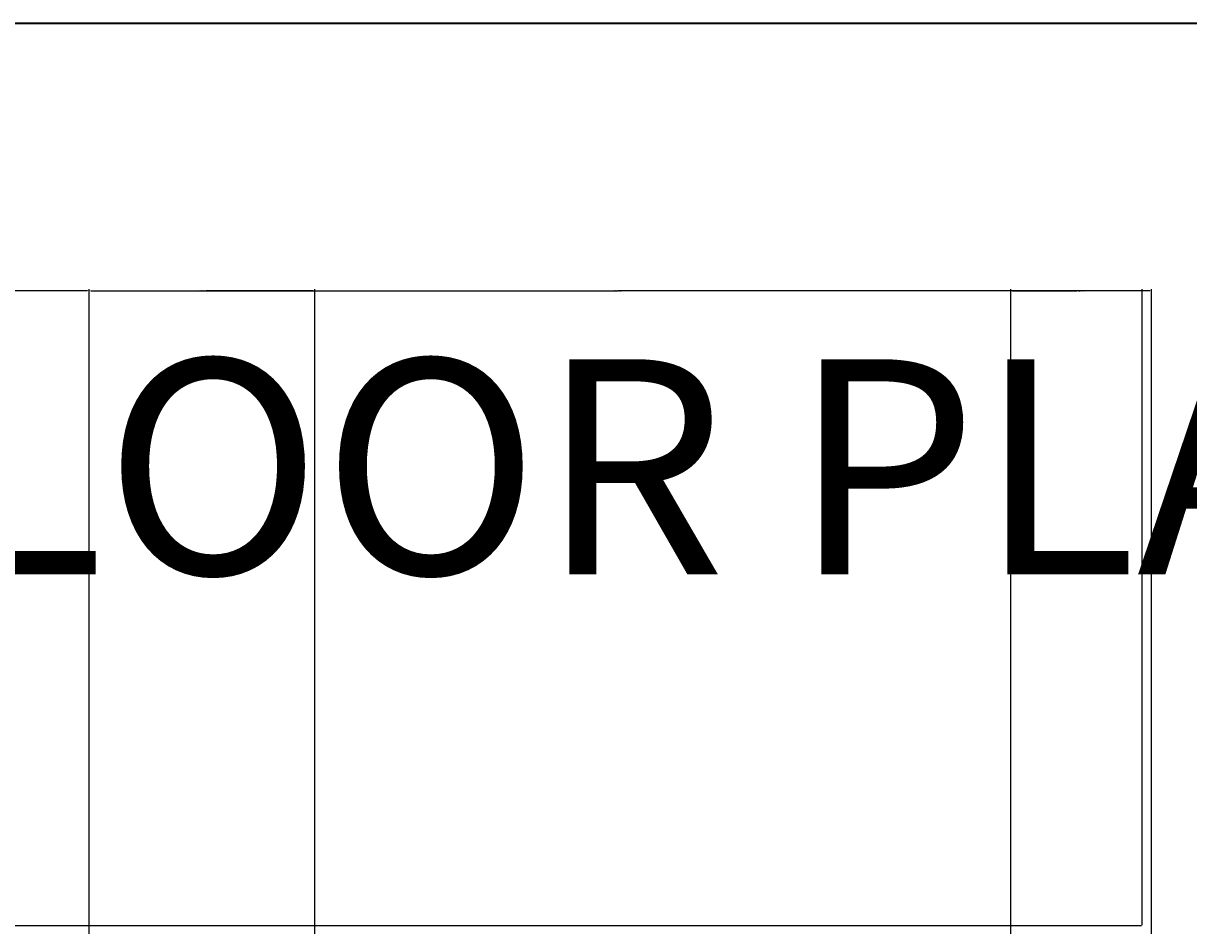
# Model space of a CAD drawing. Units: feet. Extents: x 100807 to 101423, y 154875 to 156331.
# Tile 7 of 8: x 101051 to 101176, y 156235 to 156331. Entities that reach past the tile are written whole.
import ezdxf

# ---------------------------------------------------------------- set-up
doc = ezdxf.new("R2010")
doc.units = ezdxf.units.FT
for name, color, linetype, lineweight in [('A-ANNO-DIMS', 2, 'Continuous', 18), ('A-ANNO-TITL', 7, 'Continuous', 35), ('A-ANNO-TTLB', 7, 'Continuous', 35)]:
    doc.layers.add(name, color=color, linetype=linetype, lineweight=lineweight)
doc.styles.get("Standard").update_dxf_attribs({"font": 'arial.ttf'})
doc.dimstyles.get("Standard").update_dxf_attribs({"dimtxt": 0.18, "dimasz": 0.18, "dimexe": 0.18, "dimexo": 0.0625, "dimgap": 0.09, "dimtad": 0, "dimtih": 1, "dimtoh": 1, "dimdec": 4, "dimzin": 0, "dimdsep": 46, "dimtxsty": 'Standard', "dimcen": 0.09, "dimadec": 0, "dimazin": 0, "dimtfac": 1, "dimtdec": 4, "dimtofl": 0, "dimtmove": 0, "dimatfit": 3, "dimfxl": 1, "dimtolj": 1, "dimtzin": 0, "dimarcsym": 0})

# ---------------------------------------------------------------- blocks, each defined once
blk = doc.blocks.new('*D36')
at = {"layer": 'A-ANNO-DIMS', "color": 0, "lineweight": -2, "transparency": 16777216}
for p, q in [((101058.16, 155866.64), (101058.16, 156302.91)), ((101058.34, 156302.73), (101114.88, 156302.73)), ((101171.98, 156302.73), (101115.44, 156302.73)), ((101172.16, 155866.64), (101172.16, 156302.91))]:
    blk.add_line(p, q, dxfattribs=at)
at = {"layer": 'A-ANNO-DIMS', "color": 0, "transparency": 16777216}
for points in [[(101058.34, 156302.76), (101058.34, 156302.7), (101058.16, 156302.73)], [(101171.98, 156302.76), (101171.98, 156302.7), (101172.16, 156302.73)]]:
    blk.add_solid(points, dxfattribs=at)
at = {"layer": 'Defpoints', "color": 0, "transparency": 16777216}
for p in [(101172.16, 156302.73), (101058.16, 155866.58), (101172.16, 155866.58)]:
    blk.add_point(p, dxfattribs=at)
at = {"layer": 'A-ANNO-DIMS', "color": 0, "transparency": 16777216, "insert": (101115.16, 156302.73), "char_height": 0.18, "attachment_point": 5}
blk.add_mtext('\\A1;114', dxfattribs=at)
blk = doc.blocks.new('*D38')
at = {"layer": 'A-ANNO-DIMS', "color": 0, "lineweight": -2, "transparency": 16777216}
for p, q in [((100875.16, 156234.64), (100875.16, 156302.91)), ((100875.34, 156302.73), (100966.38, 156302.73)), ((101057.98, 156302.73), (100966.94, 156302.73)), ((101058.16, 156234.64), (101058.16, 156302.91))]:
    blk.add_line(p, q, dxfattribs=at)
at = {"layer": 'A-ANNO-DIMS', "color": 0, "transparency": 16777216}
for points in [[(100875.34, 156302.76), (100875.34, 156302.7), (100875.16, 156302.73)], [(101057.98, 156302.76), (101057.98, 156302.7), (101058.16, 156302.73)]]:
    blk.add_solid(points, dxfattribs=at)
at = {"layer": 'Defpoints', "color": 0, "transparency": 16777216}
for p in [(101058.16, 156302.73), (100875.16, 156234.58), (101058.16, 156234.58)]:
    blk.add_point(p, dxfattribs=at)
at = {"layer": 'A-ANNO-DIMS', "color": 0, "transparency": 16777216, "insert": (100966.66, 156302.73), "char_height": 0.18, "attachment_point": 5}
blk.add_mtext('\\A1;183', dxfattribs=at)
blk = doc.blocks.new('*D39')
at = {"layer": 'A-ANNO-DIMS', "color": 0, "lineweight": -2, "transparency": 16777216}
for p, q in [((101058.16, 156234.64), (101058.16, 156302.91)), ((101058.34, 156302.73), (101114.38, 156302.73)), ((101170.98, 156302.73), (101114.94, 156302.73)), ((101171.16, 156234.64), (101171.16, 156302.91))]:
    blk.add_line(p, q, dxfattribs=at)
at = {"layer": 'A-ANNO-DIMS', "color": 0, "transparency": 16777216}
for points in [[(101058.34, 156302.76), (101058.34, 156302.7), (101058.16, 156302.73)], [(101170.98, 156302.76), (101170.98, 156302.7), (101171.16, 156302.73)]]:
    blk.add_solid(points, dxfattribs=at)
at = {"layer": 'Defpoints', "color": 0, "transparency": 16777216}
for p in [(101171.16, 156302.73), (101058.16, 156234.58), (101171.16, 156234.58)]:
    blk.add_point(p, dxfattribs=at)
at = {"layer": 'A-ANNO-DIMS', "color": 0, "transparency": 16777216, "insert": (101114.66, 156302.73), "char_height": 0.18, "attachment_point": 5}
blk.add_mtext('\\A1;113', dxfattribs=at)
blk = doc.blocks.new('*D40')
at = {"layer": 'A-ANNO-DIMS', "color": 0, "lineweight": -2, "transparency": 16777216}
for p, q in [((101171.09, 156234.58), (100806.83, 156234.58)), ((100807.01, 156234.4), (100807.01, 156200.26)), ((100807.01, 156165.76), (100807.01, 156199.9)), ((101171.09, 156165.58), (100806.83, 156165.58))]:
    blk.add_line(p, q, dxfattribs=at)
at = {"layer": 'A-ANNO-DIMS', "color": 0, "transparency": 16777216}
for points in [[(100806.98, 156234.4), (100807.04, 156234.4), (100807.01, 156234.58)], [(100806.98, 156165.76), (100807.04, 156165.76), (100807.01, 156165.58)]]:
    blk.add_solid(points, dxfattribs=at)
at = {"layer": 'Defpoints', "color": 0, "transparency": 16777216}
for p in [(100807.01, 156234.58), (101171.16, 156234.58), (101171.16, 156165.58)]:
    blk.add_point(p, dxfattribs=at)
at = {"layer": 'A-ANNO-DIMS', "color": 0, "transparency": 16777216, "insert": (100807.01, 156200.08), "char_height": 0.18, "attachment_point": 5}
blk.add_mtext('\\A1;69', dxfattribs=at)
blk = doc.blocks.new('*D49')
at = {"layer": 'A-ANNO-DIMS', "color": 0, "lineweight": -2, "transparency": 16777216}
for p, q in [((101157.08, 155866.64), (101157.08, 156302.91)), ((101157.26, 156302.73), (101164.16, 156302.73)), ((101171.98, 156302.73), (101165.07, 156302.73)), ((101172.16, 155866.64), (101172.16, 156302.91))]:
    blk.add_line(p, q, dxfattribs=at)
at = {"layer": 'A-ANNO-DIMS', "color": 0, "transparency": 16777216}
for points in [[(101157.26, 156302.76), (101157.26, 156302.7), (101157.08, 156302.73)], [(101171.98, 156302.76), (101171.98, 156302.7), (101172.16, 156302.73)]]:
    blk.add_solid(points, dxfattribs=at)
at = {"layer": 'Defpoints', "color": 0, "transparency": 16777216}
for p in [(101172.16, 156302.73), (101157.08, 155866.58), (101172.16, 155866.58)]:
    blk.add_point(p, dxfattribs=at)
at = {"layer": 'A-ANNO-DIMS', "color": 0, "transparency": 16777216, "insert": (101164.62, 156302.73), "char_height": 0.18, "attachment_point": 5}
blk.add_mtext('\\A1;15.075', dxfattribs=at)
blk = doc.blocks.new('*D50')
at = {"layer": 'A-ANNO-DIMS', "color": 0, "lineweight": -2, "transparency": 16777216}
for p, q in [((101058.16, 156165.64), (101058.16, 156302.91)), ((101058.34, 156302.73), (101069.79, 156302.73)), ((101082.18, 156302.73), (101070.72, 156302.73)), ((101082.36, 156165.64), (101082.36, 156302.91))]:
    blk.add_line(p, q, dxfattribs=at)
at = {"layer": 'A-ANNO-DIMS', "color": 0, "transparency": 16777216}
for points in [[(101058.34, 156302.76), (101058.34, 156302.7), (101058.16, 156302.73)], [(101082.18, 156302.76), (101082.18, 156302.7), (101082.36, 156302.73)]]:
    blk.add_solid(points, dxfattribs=at)
at = {"layer": 'Defpoints', "color": 0, "transparency": 16777216}
for p in [(101082.36, 156302.73), (101058.16, 156165.58), (101082.36, 156165.58)]:
    blk.add_point(p, dxfattribs=at)
at = {"layer": 'A-ANNO-DIMS', "color": 0, "transparency": 16777216, "insert": (101070.26, 156302.73), "char_height": 0.18, "attachment_point": 5}
blk.add_mtext('\\A1;24.205', dxfattribs=at)

msp = doc.modelspace()

# ---------------------------------------------------------------- linework, layer by layer
at = {"layer": 'A-ANNO-TTLB'}
msp.add_lwpolyline([(100830.3877, 156331.4447), (101396.4426, 156331.4447), (101396.4426, 154875.4601), (100830.3877, 154875.4601)], close=True, dxfattribs=at)

# ---------------------------------------------------------------- texts
at = {"layer": 'A-ANNO-TITL'}
msp.add_text('FLOOR PLAN', height=23.08638, dxfattribs=at).set_placement((101025.2804, 156272.2968))

# ---------------------------------------------------------------- dimensions: what is measured, and where the dimension line sits
at = {"layer": 'A-ANNO-DIMS'}
for base, p1, p2, override, picture, middle in [((101058.1564, 156302.7277), (100875.1564, 156234.5777), (101058.1564, 156234.5777), {"dimdec": 0, "dimlfac": 1, "dimrnd": 0, "dimzin": 0, "dimdsep": 46, "dimlunit": 2}, '*D38', (100966.6564, 156302.7277)), ((101172.1564, 156302.7277), (101058.1564, 155866.5789), (101172.1564, 155866.5789), {"dimdec": 0, "dimlfac": 1, "dimrnd": 0, "dimzin": 0, "dimdsep": 46, "dimlunit": 2}, '*D36', (101115.1564, 156302.7277)), ((101171.1564, 156302.7277), (101058.1564, 156234.5777), (101171.1564, 156234.5777), {"dimdec": 0, "dimlfac": 1, "dimrnd": 0, "dimzin": 0, "dimdsep": 46, "dimlunit": 2}, '*D39', (101114.6564, 156302.7277)), ((101082.3615, 156302.7277), (101058.1564, 156165.5789), (101082.3615, 156165.5789), {"dimdec": 3, "dimlfac": 1, "dimrnd": 0, "dimzin": 0, "dimdsep": 46, "dimlunit": 2}, '*D50', (101070.259, 156302.7277)), ((101172.1564, 156302.7277), (101157.0816, 155866.5789), (101172.1564, 155866.5789), {"dimdec": 3, "dimlfac": 1, "dimrnd": 0, "dimzin": 0, "dimdsep": 46, "dimlunit": 2}, '*D49', (101164.619, 156302.7277))]:
    dim = msp.add_linear_dim(base=base, p1=p1, p2=p2, dimstyle='Standard', override=override, dxfattribs=at)
    dim.commit()
    dim.dimension.update_dxf_attribs({"geometry": picture, "text_midpoint": middle})
dim = msp.add_linear_dim(base=(100807.0064, 156234.5777), p1=(101171.1564, 156165.5789), p2=(101171.1564, 156234.5777), angle=90, dimstyle='Standard', override={"dimdec": 0, "dimlfac": 1, "dimrnd": 0, "dimzin": 0, "dimdsep": 46, "dimlunit": 2}, dxfattribs=at)
dim.commit()
dim.dimension.update_dxf_attribs({"geometry": '*D40', "text_midpoint": (100807.0064, 156200.0783)})

doc.saveas('drawing.dxf')
